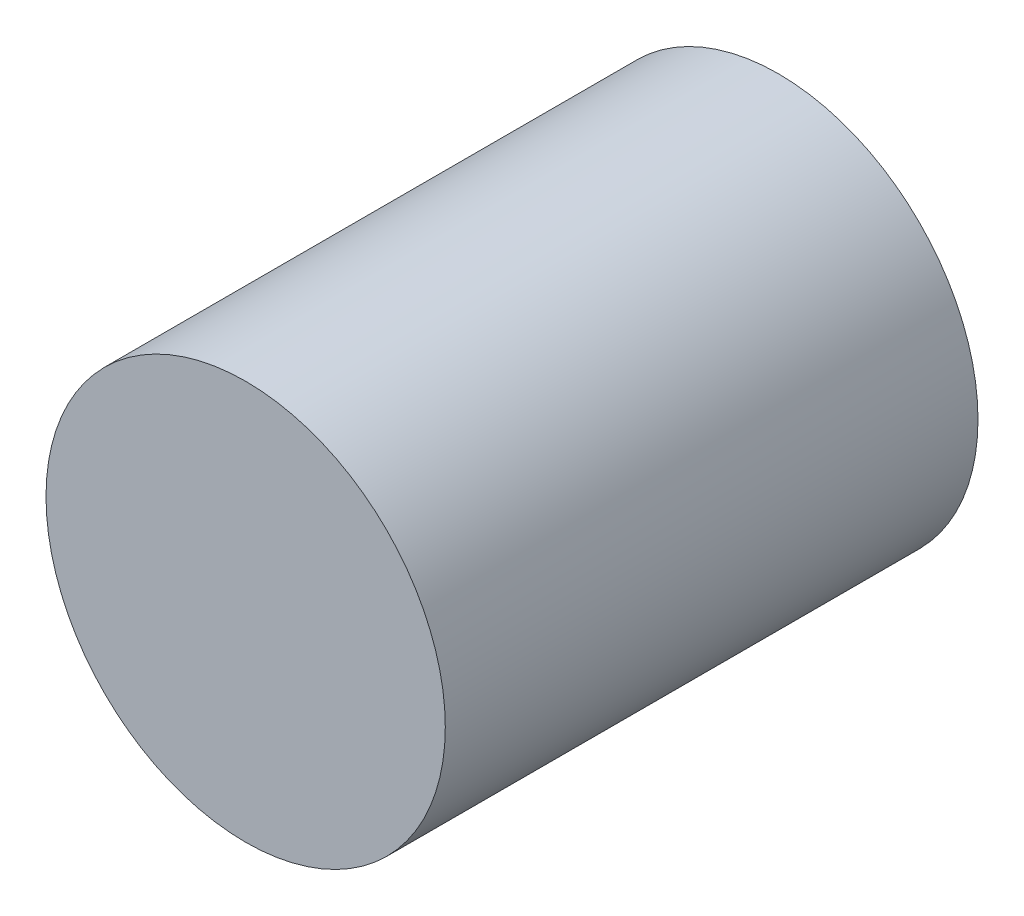
ISO-10303-21;
HEADER;
FILE_DESCRIPTION(('STEP AP214'),'2;1');
FILE_NAME('part.step','',(''),(''),'','','');
FILE_SCHEMA(('AUTOMOTIVE_DESIGN { 1 0 10303 214 1 1 1 1 }'));
ENDSEC;
DATA;
#1=APPLICATION_CONTEXT('core data for automotive mechanical design processes');
#2=APPLICATION_PROTOCOL_DEFINITION('international standard','automotive_design',2000,#1);
#3=PRODUCT_CONTEXT('',#1,'mechanical');
#4=PRODUCT('Part','Part','',(#3));
#5=PRODUCT_RELATED_PRODUCT_CATEGORY('part','',(#4));
#6=PRODUCT_DEFINITION_FORMATION('','',#4);
#7=PRODUCT_DEFINITION_CONTEXT('part definition',#1,'design');
#8=PRODUCT_DEFINITION('design','',#6,#7);
#9=PRODUCT_DEFINITION_SHAPE('','',#8);
#10=(LENGTH_UNIT() NAMED_UNIT(*) SI_UNIT(.MILLI.,.METRE.));
#11=(NAMED_UNIT(*) PLANE_ANGLE_UNIT() SI_UNIT($,.RADIAN.));
#12=(NAMED_UNIT(*) SI_UNIT($,.STERADIAN.) SOLID_ANGLE_UNIT());
#13=UNCERTAINTY_MEASURE_WITH_UNIT(LENGTH_MEASURE(1.E-05),#10,'distance_accuracy_value','');
#14=(GEOMETRIC_REPRESENTATION_CONTEXT(3) GLOBAL_UNCERTAINTY_ASSIGNED_CONTEXT((#13)) GLOBAL_UNIT_ASSIGNED_CONTEXT((#10,
#11,#12)) REPRESENTATION_CONTEXT('',''));
#15=CARTESIAN_POINT('',(0.,0.,0.));
#16=DIRECTION('',(0.,0.,1.));
#17=DIRECTION('',(1.,0.,0.));
#18=AXIS2_PLACEMENT_3D('',#15,#16,#17);
#19=CARTESIAN_POINT('',(0.,0.,12.7));
#20=DIRECTION('',(0.,0.,-1.));
#21=DIRECTION('',(-1.,0.,0.));
#22=AXIS2_PLACEMENT_3D('',#19,#20,#21);
#23=CYLINDRICAL_SURFACE('',#22,4.76);
#24=CARTESIAN_POINT('',(0.,0.,12.7));
#25=DIRECTION('',(0.,0.,1.));
#26=DIRECTION('',(1.,0.,0.));
#27=AXIS2_PLACEMENT_3D('',#24,#25,#26);
#28=CIRCLE('',#27,4.76);
#29=CARTESIAN_POINT('',(4.76,0.,12.7));
#30=VERTEX_POINT('',#29);
#31=EDGE_CURVE('E10',#30,#30,#28,.T.);
#32=ORIENTED_EDGE('',*,*,#31,.F.);
#33=EDGE_LOOP('',(#32));
#34=FACE_BOUND('',#33,.T.);
#35=CARTESIAN_POINT('',(0.,0.,0.));
#36=DIRECTION('',(0.,0.,1.));
#37=DIRECTION('',(1.,0.,0.));
#38=AXIS2_PLACEMENT_3D('',#35,#36,#37);
#39=CIRCLE('',#38,4.76);
#40=CARTESIAN_POINT('',(4.76,0.,0.));
#41=VERTEX_POINT('',#40);
#42=EDGE_CURVE('E37',#41,#41,#39,.T.);
#43=ORIENTED_EDGE('',*,*,#42,.T.);
#44=EDGE_LOOP('',(#43));
#45=FACE_BOUND('',#44,.T.);
#46=ADVANCED_FACE('F40',(#34,#45),#23,.T.);
#47=CARTESIAN_POINT('',(0.,0.,12.7));
#48=DIRECTION('',(0.,0.,1.));
#49=DIRECTION('',(1.,0.,0.));
#50=AXIS2_PLACEMENT_3D('',#47,#48,#49);
#51=PLANE('',#50);
#52=ORIENTED_EDGE('',*,*,#31,.T.);
#53=EDGE_LOOP('',(#52));
#54=FACE_BOUND('',#53,.T.);
#55=ADVANCED_FACE('F55',(#54),#51,.T.);
#56=CARTESIAN_POINT('',(0.,0.,0.));
#57=DIRECTION('',(0.,0.,1.));
#58=DIRECTION('',(1.,0.,0.));
#59=AXIS2_PLACEMENT_3D('',#56,#57,#58);
#60=PLANE('',#59);
#61=ORIENTED_EDGE('',*,*,#42,.F.);
#62=EDGE_LOOP('',(#61));
#63=FACE_BOUND('',#62,.T.);
#64=ADVANCED_FACE('F49',(#63),#60,.F.);
#65=CLOSED_SHELL('',(#46,#55,#64));
#66=MANIFOLD_SOLID_BREP('B2',#65);
#67=ADVANCED_BREP_SHAPE_REPRESENTATION('',(#18,#66),#14);
#68=SHAPE_DEFINITION_REPRESENTATION(#9,#67);
ENDSEC;
END-ISO-10303-21;
